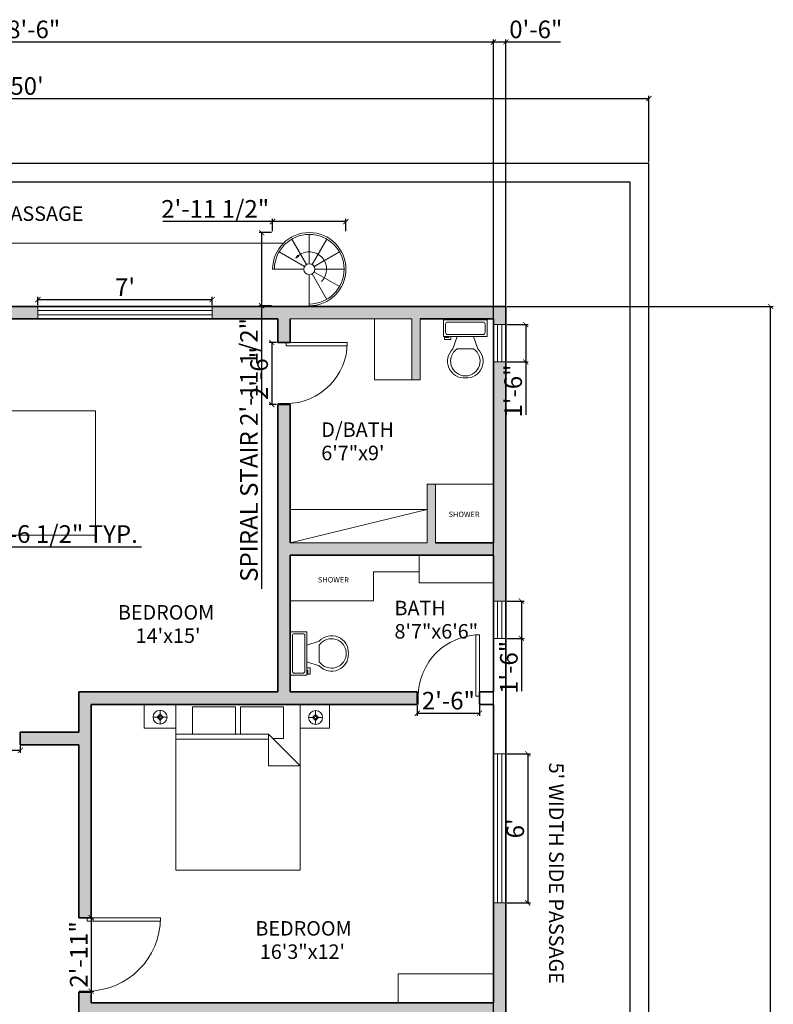
# Model space of a CAD drawing. Units: inches. Extents: x 3799 to 20199, y 1682 to 8087.
# Tile 13 of 30: x 11315 to 11679, y 2798 to 3273. Entities that reach past the tile are written whole.
import ezdxf

# ---------------------------------------------------------------- set-up
doc = ezdxf.new("R2010")
doc.units = ezdxf.units.IN
for name, color, linetype, lineweight in [('A-ANNO-DIMS', 2, 'Continuous', 18), ('A-ANNO-TEXT', 7, 'Continuous', 18), ('A-AREA-IDEN', 7, 'Continuous', 18), ('A-DOOR', 3, 'Continuous', 18), ('A-FLOR-CASE', 32, 'Continuous', 18), ('A-FLOR-FIXT', 9, 'Continuous', 18), ('A-FLOR-STRS', 41, 'Continuous', 18), ('A-FURN', 8, 'Continuous', 18), ('A-GLAZ', 152, 'Continuous', 18), ('A-WALL', 7, 'Continuous', 35), ('A-WALL-PATT', 252, 'Continuous', 13), ('C-PROP', 7, 'Continuous', 25)]:
    doc.layers.add(name, color=color, linetype=linetype, lineweight=lineweight)
doc.styles.get("Standard").update_dxf_attribs({"font": 'arial.ttf'})
doc.dimstyles.new('ISO-25', dxfattribs={"dimtxt": 8.5, "dimasz": 2.5, "dimexe": 1.25, "dimexo": 0.625, "dimtad": 1, "dimdec": 0, "dimlunit": 3, "dimtxsty": 'Standard', "dimblk": 'ARCHTICK', "dimcen": 2.5, "dimadec": 0, "dimazin": 0, "dimtfac": 1, "dimtdec": 0, "dimtmove": 0, "dimatfit": 3, "dimfxl": 1, "dimarcsym": 0})

# ---------------------------------------------------------------- blocks, each defined once
blk = doc.blocks.new('Bed - Queen')
for p, q in [((0, -80.00003), (0, 0)), ((0, 0), (59.99999, 0)), ((59.99999, 0), (59.99999, -80.00003)), ((7.99999, -1.2), (28.79998, -1.2)), ((7.99999, -14.4), (7.99999, -1.2)), ((28.79998, -1.2), (28.79998, -14.4)), ((31.19999, -1.2), (51.99999, -1.2)), ((31.19999, -14.4), (31.19999, -1.2)), ((51.99999, -1.2), (51.99999, -16.4)), ((0, -14.4), (44.8, -14.4)), ((44.8, -16.8), (0, -16.8)), ((59.99999, -29.6), (44.8, -14.4)), ((44.8, -14.4), (44.8, -29.6)), ((51.99999, -16.4), (46.79936, -16.4)), ((44.8, -29.6), (59.99999, -29.6)), ((59.99999, -80.00003), (0, -80.00003))]:
    blk.add_line(p, q)
blk = doc.blocks.new('*U59')
for p, q in [((9.5, -6), (9.5, -2)), ((-10, -8.5), (-8, -8.5)), ((-10, -9.5), (-10, -8.5)), ((-7, -9.5), (-10, -9.5)), ((-8, -8.5), (-8, -8)), ((-7, -8), (-7, -9.5)), ((-4, -8), (-6, -14)), ((4, -8), (6, -14)), ((4, -14), (-4, -14))]:
    blk.add_line(p, q)
blk.add_lwpolyline([(10.5, -8), (10.5, 0), (-10.5, 0), (-10.5, -8)], close=True)
for points in [[(-9.5, -2), (-9.5, -6)], [(8.5, -1), (-8.5, -1)], [(-8.5, -7), (8.5, -7)]]:
    blk.add_lwpolyline(points)
for centre, radius, start, end in [((-8.625, -1.875), 0.8839, 81.8699, 188.1301), ((8.625, -1.875), 0.8839, 351.8699, 98.1301), ((-8.625, -6.125), 0.8839, 171.869898, 278.1301), ((8.625, -6.125), 0.8839, 261.8699, 8.1301), ((-0.4772, -19.9188), 8.0953, 133.01722, 273.38), ((0.0374, -19.8731), 7.127, 124.50543, 269.7), ((-0.0373, -19.8731), 7.127, 270.3, 55.4946), ((0.4773, -19.9188), 8.0953, 266.62, 46.9828)]:
    blk.add_arc(centre, radius, start, end)
blk = doc.blocks.new('*U47')
for p, q in [((0, 0), (0, -100)), ((750, 0), (750, -100))]:
    blk.add_line(p, q)
blk.add_lwpolyline([(0, 0), (0, 750), (43.75, 750), (43.75, 0)], close=True)
blk.add_arc((0, 0), 750, 0, 90)
blk = doc.blocks.new('*U48')
for p, q in [((-750, 0), (-750, -100)), ((0, 0), (0, -100))]:
    blk.add_line(p, q)
blk.add_lwpolyline([(0, 0), (0, 750), (-43.75, 750), (-43.75, 0)], close=True)
blk.add_arc((0, 0), 750, 90, 180)
blk = doc.blocks.new('*U51')
for p, q in [((0, 0), (0, -100)), ((900, 0), (900, -100))]:
    blk.add_line(p, q)
blk.add_lwpolyline([(0, 0), (0, 900), (43.75, 900), (43.75, 0)], close=True)
blk.add_arc((0, 0), 900, 0, 90)
blk = doc.blocks.new('_ArchTick')
at = {"color": 0, "linetype": 'ByBlock', "const_width": 0.15}
blk.add_lwpolyline([(-0.5, -0.5), (0.5, 0.5)], dxfattribs=at)
blk = doc.blocks.new('*D65')
at = {"layer": 'A-ANNO-DIMS', "color": 0, "lineweight": -2, "transparency": 16777216}
for p, q in [((11324.12, 3135.7), (11324.12, 3139.65)), ((11324.12, 3138.4), (11408.12, 3138.4)), ((11408.12, 3135.7), (11408.12, 3139.65))]:
    blk.add_line(p, q, dxfattribs=at)
at = {"layer": 'Defpoints', "color": 0, "transparency": 16777216}
for p in [(11408.12, 3138.4), (11324.12, 3135.07), (11408.12, 3135.07)]:
    blk.add_point(p, dxfattribs=at)
at = {"layer": 'A-ANNO-DIMS', "color": 0, "lineweight": -2, "transparency": 16777216, "xscale": 2.5, "yscale": 2.5, "zscale": 2.5, "rotation": 180}
blk.add_blockref('_ArchTick', (11324.12, 3138.4), dxfattribs=at)
at = {"layer": 'A-ANNO-DIMS', "color": 0, "lineweight": -2, "transparency": 16777216, "xscale": 2.5, "yscale": 2.5, "zscale": 2.5}
blk.add_blockref('_ArchTick', (11408.12, 3138.4), dxfattribs=at)
at = {"layer": 'A-ANNO-DIMS', "color": 0, "transparency": 16777216, "insert": (11366.12, 3143.28), "char_height": 8.5, "attachment_point": 5}
blk.add_mtext("7'", dxfattribs=at)
blk = doc.blocks.new('*D66')
at = {"layer": 'A-ANNO-DIMS', "color": 0, "lineweight": -2, "transparency": 16777216}
for p, q in [((11550.48, 3126.28), (11560.66, 3126.28)), ((11559.41, 3126.28), (11559.41, 3108.28)), ((11550.48, 3108.28), (11560.66, 3108.28)), ((11559.41, 3108.28), (11559.41, 3082.73))]:
    blk.add_line(p, q, dxfattribs=at)
at = {"layer": 'Defpoints', "color": 0, "transparency": 16777216}
for p in [(11549.85, 3126.28), (11549.85, 3108.28), (11559.41, 3108.28)]:
    blk.add_point(p, dxfattribs=at)
at = {"layer": 'A-ANNO-DIMS', "color": 0, "lineweight": -2, "transparency": 16777216, "xscale": 2.5, "yscale": 2.5, "zscale": 2.5}
for p, rotation in [((11559.41, 3126.28), 90), ((11559.41, 3108.28), 270)]:
    blk.add_blockref('_ArchTick', p, dxfattribs=dict(at, rotation=rotation))
at = {"layer": 'A-ANNO-DIMS', "color": 0, "transparency": 16777216, "insert": (11554.45, 3094.25), "char_height": 8.5, "attachment_point": 5, "rotation": 90}
blk.add_mtext('1\'-6"', dxfattribs=at)
blk = doc.blocks.new('*D67')
at = {"layer": 'A-ANNO-DIMS', "color": 0, "lineweight": -2, "transparency": 16777216}
for p, q in [((11550.48, 2992.92), (11558.6, 2992.92)), ((11557.35, 2992.92), (11557.35, 2974.92)), ((11550.48, 2974.92), (11558.6, 2974.92)), ((11557.35, 2974.92), (11557.35, 2949.38))]:
    blk.add_line(p, q, dxfattribs=at)
at = {"layer": 'Defpoints', "color": 0, "transparency": 16777216}
for p in [(11549.85, 2992.92), (11549.85, 2974.92), (11557.35, 2974.92)]:
    blk.add_point(p, dxfattribs=at)
at = {"layer": 'A-ANNO-DIMS', "color": 0, "lineweight": -2, "transparency": 16777216, "xscale": 2.5, "yscale": 2.5, "zscale": 2.5}
for p, rotation in [((11557.35, 2992.92), 90), ((11557.35, 2974.92), 270)]:
    blk.add_blockref('_ArchTick', p, dxfattribs=dict(at, rotation=rotation))
at = {"layer": 'A-ANNO-DIMS', "color": 0, "transparency": 16777216, "insert": (11552.38, 2960.9), "char_height": 8.5, "attachment_point": 5, "rotation": 90}
blk.add_mtext('1\'-6"', dxfattribs=at)
blk = doc.blocks.new('*D68')
at = {"layer": 'A-ANNO-DIMS', "color": 0, "lineweight": -2, "transparency": 16777216}
for p, q in [((11550.48, 2919.23), (11561.66, 2919.23)), ((11560.41, 2919.23), (11560.41, 2847.23)), ((11550.48, 2847.23), (11561.66, 2847.23))]:
    blk.add_line(p, q, dxfattribs=at)
at = {"layer": 'Defpoints', "color": 0, "transparency": 16777216}
for p in [(11549.85, 2919.23), (11549.85, 2847.23), (11560.41, 2847.23)]:
    blk.add_point(p, dxfattribs=at)
at = {"layer": 'A-ANNO-DIMS', "color": 0, "lineweight": -2, "transparency": 16777216, "xscale": 2.5, "yscale": 2.5, "zscale": 2.5}
for p, rotation in [((11560.41, 2919.23), 90), ((11560.41, 2847.23), 270)]:
    blk.add_blockref('_ArchTick', p, dxfattribs=dict(at, rotation=rotation))
at = {"layer": 'A-ANNO-DIMS', "color": 0, "transparency": 16777216, "insert": (11555.45, 2883.23), "char_height": 8.5, "attachment_point": 5, "rotation": 90}
blk.add_mtext("6'", dxfattribs=at)
blk = doc.blocks.new('*D78')
at = {"layer": 'A-ANNO-DIMS', "color": 0, "lineweight": -2, "transparency": 16777216}
for p, q in [((11018.85, 3204.7), (11018.85, 3236.64)), ((11618.85, 3204.7), (11618.85, 3236.64)), ((11018.85, 3235.39), (11618.85, 3235.39))]:
    blk.add_line(p, q, dxfattribs=at)
at = {"layer": 'Defpoints', "color": 0, "transparency": 16777216}
for p in [(11618.85, 3235.39), (11018.85, 3204.07), (11618.85, 3204.07)]:
    blk.add_point(p, dxfattribs=at)
at = {"layer": 'A-ANNO-DIMS', "color": 0, "lineweight": -2, "transparency": 16777216, "xscale": 2.5, "yscale": 2.5, "zscale": 2.5, "rotation": 180}
blk.add_blockref('_ArchTick', (11018.85, 3235.39), dxfattribs=at)
at = {"layer": 'A-ANNO-DIMS', "color": 0, "lineweight": -2, "transparency": 16777216, "xscale": 2.5, "yscale": 2.5, "zscale": 2.5}
blk.add_blockref('_ArchTick', (11618.85, 3235.39), dxfattribs=at)
at = {"layer": 'A-ANNO-DIMS', "color": 0, "transparency": 16777216, "insert": (11318.85, 3240.35), "char_height": 8.5, "attachment_point": 5}
blk.add_mtext("50'", dxfattribs=at)
blk = doc.blocks.new('*D84')
at = {"layer": 'A-ANNO-DIMS', "color": 0, "lineweight": -2, "transparency": 16777216}
for p, q in [((11344.48, 2840.12), (11351.04, 2840.12)), ((11349.79, 2840.12), (11349.79, 2804.68)), ((11344.48, 2804.68), (11351.04, 2804.68))]:
    blk.add_line(p, q, dxfattribs=at)
at = {"layer": 'Defpoints', "color": 0, "transparency": 16777216}
for p in [(11343.85, 2840.12), (11343.85, 2804.68), (11349.79, 2804.68)]:
    blk.add_point(p, dxfattribs=at)
at = {"layer": 'A-ANNO-DIMS', "color": 0, "lineweight": -2, "transparency": 16777216, "xscale": 2.5, "yscale": 2.5, "zscale": 2.5}
for p, rotation in [((11349.79, 2840.12), 90), ((11349.79, 2804.68), 270)]:
    blk.add_blockref('_ArchTick', p, dxfattribs=dict(at, rotation=rotation))
at = {"layer": 'A-ANNO-DIMS', "color": 0, "transparency": 16777216, "insert": (11344.9, 2822.4), "char_height": 8.5, "attachment_point": 5, "rotation": 90}
blk.add_mtext('2\'-11"', dxfattribs=at)
blk = doc.blocks.new('*D86')
at = {"layer": 'A-ANNO-DIMS', "color": 0, "lineweight": -2, "transparency": 16777216}
for p, q in [((11279.6, 2922.98), (11279.6, 2919.65)), ((11315.6, 2922.98), (11315.6, 2919.65)), ((11279.6, 2920.9), (11315.6, 2920.9))]:
    blk.add_line(p, q, dxfattribs=at)
at = {"layer": 'Defpoints', "color": 0, "transparency": 16777216}
for p in [(11279.6, 2923.61), (11315.6, 2923.61), (11315.6, 2920.9)]:
    blk.add_point(p, dxfattribs=at)
at = {"layer": 'A-ANNO-DIMS', "color": 0, "lineweight": -2, "transparency": 16777216, "xscale": 2.5, "yscale": 2.5, "zscale": 2.5, "rotation": 180}
blk.add_blockref('_ArchTick', (11279.6, 2920.9), dxfattribs=at)
at = {"layer": 'A-ANNO-DIMS', "color": 0, "lineweight": -2, "transparency": 16777216, "xscale": 2.5, "yscale": 2.5, "zscale": 2.5}
blk.add_blockref('_ArchTick', (11315.6, 2920.9), dxfattribs=at)
at = {"layer": 'A-ANNO-DIMS', "color": 0, "transparency": 16777216, "insert": (11297.6, 2925.87), "char_height": 8.5, "attachment_point": 5}
blk.add_mtext("3'", dxfattribs=at)
blk = doc.blocks.new('*D88')
at = {"layer": 'A-ANNO-DIMS', "color": 0, "lineweight": -2, "transparency": 16777216}
for p, q in [((11507.11, 2942.45), (11507.11, 2937.53)), ((11537.11, 2942.45), (11537.11, 2937.53)), ((11507.11, 2938.78), (11537.11, 2938.78))]:
    blk.add_line(p, q, dxfattribs=at)
at = {"layer": 'Defpoints', "color": 0, "transparency": 16777216}
for p in [(11507.11, 2943.07), (11537.11, 2943.07), (11537.11, 2938.78)]:
    blk.add_point(p, dxfattribs=at)
at = {"layer": 'A-ANNO-DIMS', "color": 0, "lineweight": -2, "transparency": 16777216, "xscale": 2.5, "yscale": 2.5, "zscale": 2.5, "rotation": 180}
blk.add_blockref('_ArchTick', (11507.11, 2938.78), dxfattribs=at)
at = {"layer": 'A-ANNO-DIMS', "color": 0, "lineweight": -2, "transparency": 16777216, "xscale": 2.5, "yscale": 2.5, "zscale": 2.5}
blk.add_blockref('_ArchTick', (11537.11, 2938.78), dxfattribs=at)
at = {"layer": 'A-ANNO-DIMS', "color": 0, "transparency": 16777216, "insert": (11522.11, 2943.74), "char_height": 8.5, "attachment_point": 5}
blk.add_mtext('2\'-6"', dxfattribs=at)
blk = doc.blocks.new('*D89')
at = {"layer": 'A-ANNO-DIMS', "color": 0, "lineweight": -2, "transparency": 16777216}
for p, q in [((11439.23, 3117.71), (11435.63, 3117.71)), ((11436.88, 3117.71), (11436.88, 3087.71)), ((11439.23, 3087.71), (11435.63, 3087.71))]:
    blk.add_line(p, q, dxfattribs=at)
at = {"layer": 'Defpoints', "color": 0, "transparency": 16777216}
for p in [(11439.85, 3117.71), (11436.88, 3087.71), (11439.85, 3087.71)]:
    blk.add_point(p, dxfattribs=at)
at = {"layer": 'A-ANNO-DIMS', "color": 0, "lineweight": -2, "transparency": 16777216, "xscale": 2.5, "yscale": 2.5, "zscale": 2.5}
for p, rotation in [((11436.88, 3117.71), 90), ((11436.88, 3087.71), 270)]:
    blk.add_blockref('_ArchTick', p, dxfattribs=dict(at, rotation=rotation))
at = {"layer": 'A-ANNO-DIMS', "color": 0, "transparency": 16777216, "insert": (11431.91, 3102.71), "char_height": 8.5, "attachment_point": 5, "rotation": 90}
blk.add_mtext('2\'-6"', dxfattribs=at)
blk = doc.blocks.new('Lamp - Table')
for p, q in [((-1, 0), (-7, 0)), ((0, 3), (-3, 0)), ((-3, 0), (0, -3)), ((0, 7), (0, 1)), ((3, 0), (0, 3)), ((0, -3), (3, 0)), ((1, 0), (7, 0)), ((0, -1), (0, -7))]:
    blk.add_line(p, q)
for radius in [7, 1]:
    blk.add_circle((0, 0), radius)
blk = doc.blocks.new('Staircase - Spiral')
for p, q in [((-2.2579, 3.91), (-14.25, 24.681)), ((0, 4.5), (0, 30)), ((-3.8566, 2.226), (-24.6818, 14.25)), ((-4.5, 0), (-28.5, 0)), ((4.5, 0), (30, 0)), ((-3.8954, -2.2492), (-24.6818, -14.2502)), ((-2.2755, -3.9415), (-14.25, -24.6819)), ((0, -4.5002), (0, -28.5002)), ((2.2614, -3.9171), (14.25, -24.6819)), ((3.8999, -2.2518), (24.6817, -14.2502)), ((8.5, -10.5002), (11, -9.0002)), ((9, -11.0002), (8.5, -10.5002)), ((9, -11.0002), (9.5, -11.5002)), ((11, -9.0002), (9.5, -11.5002))]:
    blk.add_line(p, q)
blk.add_circle((0, 0), 4.5)
for radius, start, end in [(30, 90, 0), (28.5, 90, 0), (14.2215, 135, 309.2894)]:
    blk.add_arc((0, 0), radius, start, end)
blk = doc.blocks.new('WIN-84IN-6IN-FRAME')
for p, q in [((0, 84), (6, 84)), ((2, 0), (2, 84)), ((4, 0), (4, 84)), ((0, 0), (6, 0))]:
    blk.add_line(p, q)
blk = doc.blocks.new('WIN-18IN-6IN-FRAME')
for p, q in [((0, 18), (6, 18)), ((2, 0), (2, 18)), ((4, 0), (4, 18)), ((0, 0), (6, 0))]:
    blk.add_line(p, q)
blk = doc.blocks.new('*D246')
at = {"layer": 'A-ANNO-DIMS', "color": 0, "lineweight": -2, "transparency": 16777216}
for p, q in [((11256.67, 3019.5), (11256.67, 3017.87)), ((11256.67, 3019.12), (11263.41, 3019.12)), ((11263.41, 3019.5), (11263.41, 3017.87)), ((11263.41, 3019.12), (11374.03, 3019.12))]:
    blk.add_line(p, q, dxfattribs=at)
at = {"layer": 'Defpoints', "color": 0, "transparency": 16777216}
for p in [(11256.67, 3020.13), (11263.41, 3020.13), (11263.41, 3019.12)]:
    blk.add_point(p, dxfattribs=at)
at = {"layer": 'A-ANNO-DIMS', "color": 0, "lineweight": -2, "transparency": 16777216, "xscale": 2.5, "yscale": 2.5, "zscale": 2.5, "rotation": 180}
blk.add_blockref('_ArchTick', (11256.67, 3019.12), dxfattribs=at)
at = {"layer": 'A-ANNO-DIMS', "color": 0, "lineweight": -2, "transparency": 16777216, "xscale": 2.5, "yscale": 2.5, "zscale": 2.5}
blk.add_blockref('_ArchTick', (11263.41, 3019.12), dxfattribs=at)
at = {"layer": 'A-ANNO-DIMS', "color": 0, "transparency": 16777216, "insert": (11319.97, 3024.14), "char_height": 8.5, "attachment_point": 5}
blk.add_mtext('LAMP 0\'-6 1/2" TYP.', dxfattribs=at)
blk = doc.blocks.new('*D350')
at = {"layer": 'A-ANNO-DIMS', "color": 0, "lineweight": -2, "transparency": 16777216}
for p, q in [((11436.7, 3170.72), (11430.77, 3170.72)), ((11432.02, 3170.72), (11432.02, 3135.36)), ((11436.7, 3135.36), (11430.77, 3135.36)), ((11432.02, 3135.36), (11432.02, 2998.84))]:
    blk.add_line(p, q, dxfattribs=at)
at = {"layer": 'Defpoints', "color": 0, "transparency": 16777216}
for p in [(11437.32, 3170.72), (11432.02, 3135.36), (11437.32, 3135.36)]:
    blk.add_point(p, dxfattribs=at)
at = {"layer": 'A-ANNO-DIMS', "color": 0, "lineweight": -2, "transparency": 16777216, "xscale": 2.5, "yscale": 2.5, "zscale": 2.5}
for p, rotation in [((11432.02, 3170.72), 90), ((11432.02, 3135.36), 270)]:
    blk.add_blockref('_ArchTick', p, dxfattribs=dict(at, rotation=rotation))
at = {"layer": 'A-ANNO-DIMS', "color": 0, "transparency": 16777216, "insert": (11427, 3065.85), "char_height": 8.5, "attachment_point": 5, "rotation": 90}
blk.add_mtext('SPIRAL STAIR 2\'-11 1/2"', dxfattribs=at)
blk = doc.blocks.new('*D351')
at = {"layer": 'A-ANNO-DIMS', "color": 0, "lineweight": -2, "transparency": 16777216}
for p, q in [((11437.32, 3176.02), (11384.42, 3176.02)), ((11437.32, 3171.34), (11437.32, 3177.27)), ((11472.68, 3176.02), (11437.32, 3176.02)), ((11472.68, 3171.34), (11472.68, 3177.27))]:
    blk.add_line(p, q, dxfattribs=at)
at = {"layer": 'Defpoints', "color": 0, "transparency": 16777216}
for p in [(11437.32, 3176.02), (11437.32, 3170.72), (11472.68, 3170.72)]:
    blk.add_point(p, dxfattribs=at)
at = {"layer": 'A-ANNO-DIMS', "color": 0, "lineweight": -2, "transparency": 16777216, "xscale": 2.5, "yscale": 2.5, "zscale": 2.5, "rotation": 180}
blk.add_blockref('_ArchTick', (11437.32, 3176.02), dxfattribs=at)
at = {"layer": 'A-ANNO-DIMS', "color": 0, "lineweight": -2, "transparency": 16777216, "xscale": 2.5, "yscale": 2.5, "zscale": 2.5}
blk.add_blockref('_ArchTick', (11472.68, 3176.02), dxfattribs=at)
at = {"layer": 'A-ANNO-DIMS', "color": 0, "transparency": 16777216, "insert": (11409.62, 3181.04), "char_height": 8.5, "attachment_point": 5}
blk.add_mtext('2\'-11 1/2"', dxfattribs=at)
blk = doc.blocks.new('*D371')
at = {"layer": 'A-ANNO-DIMS', "color": 0, "lineweight": -2, "transparency": 16777216}
for p, q in [((11543.85, 3126.9), (11543.85, 3263.92)), ((11549.85, 3126.9), (11549.85, 3263.92)), ((11543.85, 3262.67), (11549.85, 3262.67)), ((11549.85, 3262.67), (11576.2, 3262.67))]:
    blk.add_line(p, q, dxfattribs=at)
at = {"layer": 'Defpoints', "color": 0, "transparency": 16777216}
for p in [(11549.85, 3262.67), (11543.85, 3126.28), (11549.85, 3126.28)]:
    blk.add_point(p, dxfattribs=at)
at = {"layer": 'A-ANNO-DIMS', "color": 0, "lineweight": -2, "transparency": 16777216, "xscale": 2.5, "yscale": 2.5, "zscale": 2.5, "rotation": 180}
blk.add_blockref('_ArchTick', (11543.85, 3262.67), dxfattribs=at)
at = {"layer": 'A-ANNO-DIMS', "color": 0, "lineweight": -2, "transparency": 16777216, "xscale": 2.5, "yscale": 2.5, "zscale": 2.5}
blk.add_blockref('_ArchTick', (11549.85, 3262.67), dxfattribs=at)
at = {"layer": 'A-ANNO-DIMS', "color": 0, "transparency": 16777216, "insert": (11564.28, 3267.64), "char_height": 8.5, "attachment_point": 5}
blk.add_mtext('0\'-6"', dxfattribs=at)
blk = doc.blocks.new('*D372')
at = {"layer": 'A-ANNO-DIMS', "color": 0, "lineweight": -2, "transparency": 16777216}
for p, q in [((11543.85, 2537.7), (11543.85, 3263.92)), ((11549.85, 2537.7), (11549.85, 3263.92)), ((11543.85, 3262.67), (11549.85, 3262.67)), ((11549.85, 3262.67), (11576.2, 3262.67))]:
    blk.add_line(p, q, dxfattribs=at)
at = {"layer": 'Defpoints', "color": 0, "transparency": 16777216}
for p in [(11549.85, 3262.67), (11543.85, 2537.07), (11549.85, 2537.07)]:
    blk.add_point(p, dxfattribs=at)
at = {"layer": 'A-ANNO-DIMS', "color": 0, "lineweight": -2, "transparency": 16777216, "xscale": 2.5, "yscale": 2.5, "zscale": 2.5, "rotation": 180}
blk.add_blockref('_ArchTick', (11543.85, 3262.67), dxfattribs=at)
at = {"layer": 'A-ANNO-DIMS', "color": 0, "lineweight": -2, "transparency": 16777216, "xscale": 2.5, "yscale": 2.5, "zscale": 2.5}
blk.add_blockref('_ArchTick', (11549.85, 3262.67), dxfattribs=at)
at = {"layer": 'A-ANNO-DIMS', "color": 0, "transparency": 16777216, "insert": (11564.28, 3267.64), "char_height": 8.5, "attachment_point": 5}
blk.add_mtext('0\'-6"', dxfattribs=at)
blk = doc.blocks.new('*D373')
at = {"layer": 'A-ANNO-DIMS', "color": 0, "lineweight": -2, "transparency": 16777216}
for p, q in [((11087.85, 3135.7), (11087.85, 3263.92)), ((11549.85, 3135.7), (11549.85, 3263.92)), ((11087.85, 3262.67), (11549.85, 3262.67))]:
    blk.add_line(p, q, dxfattribs=at)
at = {"layer": 'Defpoints', "color": 0, "transparency": 16777216}
for p in [(11549.85, 3262.67), (11087.85, 3135.07), (11549.85, 3135.07)]:
    blk.add_point(p, dxfattribs=at)
at = {"layer": 'A-ANNO-DIMS', "color": 0, "lineweight": -2, "transparency": 16777216, "xscale": 2.5, "yscale": 2.5, "zscale": 2.5, "rotation": 180}
blk.add_blockref('_ArchTick', (11087.85, 3262.67), dxfattribs=at)
at = {"layer": 'A-ANNO-DIMS', "color": 0, "lineweight": -2, "transparency": 16777216, "xscale": 2.5, "yscale": 2.5, "zscale": 2.5}
blk.add_blockref('_ArchTick', (11549.85, 3262.67), dxfattribs=at)
at = {"layer": 'A-ANNO-DIMS', "color": 0, "transparency": 16777216, "insert": (11318.85, 3267.64), "char_height": 8.5, "attachment_point": 5}
blk.add_mtext('38\'-6"', dxfattribs=at)
blk = doc.blocks.new('*D374')
at = {"layer": 'A-ANNO-DIMS', "color": 0, "lineweight": -2, "transparency": 16777216}
for p, q in [((11550.48, 3135.07), (11678.7, 3135.07)), ((11677.45, 2325.07), (11677.45, 3135.07)), ((11550.48, 2325.07), (11678.7, 2325.07))]:
    blk.add_line(p, q, dxfattribs=at)
at = {"layer": 'Defpoints', "color": 0, "transparency": 16777216}
for p in [(11549.85, 3135.07), (11677.45, 3135.07), (11549.85, 2325.07)]:
    blk.add_point(p, dxfattribs=at)
at = {"layer": 'A-ANNO-DIMS', "color": 0, "lineweight": -2, "transparency": 16777216, "xscale": 2.5, "yscale": 2.5, "zscale": 2.5}
for p, rotation in [((11677.45, 3135.07), 90), ((11677.45, 2325.07), 270)]:
    blk.add_blockref('_ArchTick', p, dxfattribs=dict(at, rotation=rotation))
at = {"layer": 'A-ANNO-DIMS', "color": 0, "transparency": 16777216, "insert": (11672.49, 2730.07), "char_height": 8.5, "attachment_point": 5, "rotation": 90}
blk.add_mtext('67\'-6"', dxfattribs=at)

msp = doc.modelspace()

# ---------------------------------------------------------------- hatches: boundary and pattern name
at = {"layer": 'A-WALL-PATT'}
h = msp.add_hatch(color=256, dxfattribs=at)
h.dxf.hatch_style = 1
h.paths.add_polyline_path([(11549.85, 2537.07), (11543.85, 2537.07), (11543.85, 2493.07), (11500.92, 2493.07), (11500.92, 2487.07), (11543.85, 2487.07), (11543.85, 2331.07), (11512.59, 2331.07), (11512.59, 2325.07), (11549.85, 2325.07)])
h.paths.add_polyline_path([(11404.92, 2493.07), (11369.85, 2493.07), (11369.85, 2535.29), (11363.85, 2535.29), (11363.85, 2493.07), (11359.67, 2493.07), (11359.67, 2487.07), (11404.92, 2487.07)])
h.paths.add_polyline_path([(11347.67, 2493.07), (11315.85, 2493.07), (11315.85, 2481.32), (11321.85, 2481.32), (11321.85, 2487.07), (11347.67, 2487.07)])
h.paths.add_polyline_path([(11246.96, 2394.07), (11231.85, 2394.07), (11231.85, 2493.07), (11126.81, 2493.07), (11126.81, 2487.07), (11225.85, 2487.07), (11225.85, 2325.07), (11315.85, 2325.07), (11315.85, 2331.07), (11231.85, 2331.07), (11231.85, 2388.07), (11246.96, 2388.07)])
h.paths.add_polyline_path([(11368.59, 2331.07), (11321.85, 2331.07), (11321.85, 2421.32), (11319.79, 2421.32), (11315.85, 2421.32), (11315.85, 2394.07), (11306.96, 2394.07), (11306.96, 2392.01), (11306.96, 2388.07), (11315.85, 2388.07), (11315.85, 2325.07), (11368.59, 2325.07)])
h.paths.add_polyline_path([(11211.5, 2599.62), (11175.25, 2599.62), (11175.25, 2594.62), (11206.5, 2594.62), (11206.5, 2541.62), (11137.5, 2541.62), (11137.5, 2594.62), (11145.25, 2594.62), (11145.25, 2599.62), (11132.5, 2599.62), (11132.5, 2536.62), (11211.5, 2536.62)], flags=17)
h.paths.add_polyline_path([(11278.96, 2650.07), (11117.85, 2650.07), (11117.85, 2668.07), (11111.85, 2668.07), (11111.85, 2650.07), (11087.85, 2650.07), (11087.85, 2526.57), (11093.85, 2526.57), (11093.85, 2644.07), (11278.96, 2644.07)])
h.paths.add_polyline_path([(11096.81, 2491.01), (11096.81, 2493.07), (11093.85, 2493.07), (11093.85, 2496.57), (11087.85, 2496.57), (11087.85, 2487.07), (11096.81, 2487.07)])
h.paths.add_polyline_path([(11445.85, 3087.71), (11439.85, 3087.71), (11439.85, 2949.07), (11343.85, 2949.07), (11343.85, 2929.61), (11315.6, 2929.61), (11315.6, 2923.61), (11343.85, 2923.61), (11343.85, 2840.12), (11349.85, 2840.12), (11349.85, 2943.07), (11507.11, 2943.07), (11507.11, 2949.07), (11445.85, 2949.07), (11445.85, 3015.07), (11543.85, 3015.07), (11543.85, 2992.92), (11549.85, 2992.92), (11549.85, 3108.28), (11543.85, 3108.28), (11543.85, 3021.07), (11515.89, 3021.07), (11515.89, 3049.36), (11511.89, 3049.36), (11511.89, 3021.07), (11445.85, 3021.07)])
h.paths.add_polyline_path([(11549.85, 3135.07), (11408.12, 3135.07), (11408.12, 3129.07), (11439.85, 3129.07), (11439.85, 3117.71), (11443.79, 3117.71), (11445.85, 3117.71), (11445.85, 3129.07), (11504.47, 3129.07), (11504.47, 3099.65), (11508.47, 3099.65), (11508.47, 3129.07), (11543.85, 3129.07), (11543.85, 3126.28), (11549.85, 3126.28)])
h.paths.add_polyline_path([(11324.12, 3135.07), (11087.85, 3135.07), (11087.85, 3083.46), (11093.85, 3083.46), (11093.85, 3129.07), (11265.85, 3129.07), (11265.85, 3050.07), (11240.75, 3050.07), (11240.75, 3044.07), (11265.85, 3044.07), (11265.85, 2895.64), (11271.85, 2895.64), (11271.85, 2923.61), (11279.6, 2923.61), (11279.6, 2929.61), (11271.85, 2929.61), (11271.85, 3129.07), (11324.12, 3129.07)])
h.paths.add_polyline_path([(11210.75, 3050.07), (11133.85, 3050.07), (11133.85, 3088.63), (11129.85, 3088.54), (11129.85, 3050.07), (11093.85, 3050.07), (11093.85, 3059.46), (11087.85, 3059.46), (11087.85, 3030.25), (11093.85, 3030.25), (11093.85, 3044.07), (11210.75, 3044.07)], flags=17)
h.paths.add_polyline_path([(11093.85, 2982.25), (11087.85, 2982.25), (11087.85, 2913.95), (11093.85, 2913.95)], flags=17)
h.paths.add_polyline_path([(11271.85, 2859.64), (11265.85, 2859.64), (11265.85, 2854.07), (11093.85, 2854.07), (11093.85, 2865.95), (11087.85, 2865.95), (11087.85, 2848.07), (11111.85, 2848.07), (11111.85, 2812.07), (11117.85, 2812.07), (11117.85, 2848.07), (11271.85, 2848.07)])
h.paths.add_polyline_path([(11549.85, 2847.23), (11543.85, 2847.23), (11543.85, 2799.07), (11349.85, 2799.07), (11349.85, 2804.12), (11343.85, 2804.12), (11343.85, 2753.07), (11349.85, 2753.07), (11349.85, 2793.07), (11543.85, 2793.07), (11543.85, 2752.31), (11549.85, 2752.31)])
h.paths.add_polyline_path([(11549.85, 2692.31), (11543.85, 2692.31), (11543.85, 2650.07), (11343.85, 2650.07), (11338.96, 2650.07), (11338.96, 2644.07), (11349.85, 2644.07), (11363.85, 2644.07), (11363.85, 2608.29), (11369.85, 2608.29), (11369.85, 2644.07), (11543.85, 2644.07), (11543.85, 2621.07), (11549.85, 2621.07)])

# ---------------------------------------------------------------- linework, layer by layer
at = {"layer": 'A-FLOR-CASE'}
for p, q in [((11543.85, 2812.98), (11497.92, 2812.98)), ((11497.92, 2812.98), (11497.92, 2799.07))]:
    msp.add_line(p, q, dxfattribs=at)
at = {"layer": 'A-FLOR-FIXT'}
for p, q in [((11504.47, 3129.07), (11445.85, 3129.07)), ((11486.47, 3129.07), (11486.47, 3099.65)), ((11504.47, 3129.07), (11504.47, 3099.65)), ((11508.47, 3129.07), (11508.47, 3099.65)), ((11486.47, 3099.65), (11504.47, 3099.65)), ((11508.47, 3099.65), (11504.47, 3099.65)), ((11511.89, 3021.07), (11511.89, 3049.36)), ((11511.89, 3049.36), (11543.85, 3049.36)), ((11515.89, 3021.07), (11515.89, 3049.36)), ((11511.89, 3037.17), (11445.85, 3037.17)), ((11445.85, 3021.07), (11511.89, 3037.17)), ((11511.89, 3021.07), (11445.85, 3021.07)), ((11508.04, 3001.74), (11508.04, 3015.07)), ((11508.04, 3007.02), (11486.04, 3007.02)), ((11486.04, 3007.02), (11486.04, 2993.01)), ((11543.85, 3001.74), (11508.04, 3001.74)), ((11486.04, 2993.01), (11445.85, 2993.01))]:
    msp.add_line(p, q, dxfattribs=at)
at = {"layer": 'A-FLOR-STRS'}
msp.add_line((11087.85, 3165.66), (11442.62, 3165.66), dxfattribs=at)
at = {"layer": 'A-FURN'}
for points in [[(11390.6, 2943.07), (11375.38, 2943.07), (11375.38, 2931.5), (11390.6, 2931.5)], [(11450.6, 2943.07), (11464.72, 2943.07), (11464.72, 2931.5), (11450.6, 2931.5)]]:
    msp.add_lwpolyline(points, close=True, dxfattribs=at)
at = {"layer": 'A-GLAZ'}
for p, q in [((11543.85, 2919.23), (11549.85, 2919.23)), ((11545.85, 2847.23), (11545.85, 2919.23)), ((11547.85, 2847.23), (11547.85, 2919.23)), ((11543.85, 2847.23), (11549.85, 2847.23))]:
    msp.add_line(p, q, dxfattribs=at)
at = {"layer": 'A-WALL'}
for p, q in [((11549.85, 3135.07), (11087.85, 3135.07)), ((11549.85, 2325.07), (11549.85, 3135.07)), ((11439.85, 3129.07), (11271.85, 3129.07)), ((11439.85, 3129.07), (11439.85, 3117.71)), ((11445.85, 3129.07), (11445.85, 3117.71)), ((11543.85, 3129.07), (11508.47, 3129.07)), ((11543.85, 3021.07), (11543.85, 3129.07)), ((11439.85, 3117.71), (11445.85, 3117.71)), ((11439.85, 3087.71), (11445.85, 3087.71)), ((11439.85, 3087.71), (11439.85, 2949.07)), ((11445.85, 3087.71), (11445.85, 3021.07)), ((11543.85, 3021.07), (11515.89, 3021.07)), ((11543.85, 3015.07), (11445.85, 3015.07)), ((11445.85, 3015.07), (11445.85, 2949.07)), ((11543.85, 2949.07), (11543.85, 3015.07)), ((11439.85, 2949.07), (11343.85, 2949.07)), ((11343.85, 2929.61), (11343.85, 2949.07)), ((11445.85, 2949.07), (11507.11, 2949.07)), ((11507.11, 2943.07), (11507.11, 2949.07)), ((11537.11, 2943.07), (11537.11, 2949.07)), ((11537.11, 2949.07), (11543.85, 2949.07)), ((11349.85, 2840.12), (11349.85, 2943.07)), ((11507.11, 2943.07), (11349.85, 2943.07)), ((11543.85, 2943.07), (11537.11, 2943.07)), ((11543.85, 2799.07), (11543.85, 2943.07)), ((11343.85, 2929.61), (11315.6, 2929.61)), ((11315.6, 2929.61), (11315.6, 2923.61)), ((11343.85, 2923.61), (11315.6, 2923.61)), ((11343.85, 2840.12), (11343.85, 2923.61)), ((11349.85, 2840.12), (11343.85, 2840.12)), ((11349.85, 2804.12), (11343.85, 2804.12)), ((11343.85, 2753.07), (11343.85, 2804.12)), ((11349.85, 2799.07), (11349.85, 2804.12)), ((11543.85, 2799.07), (11349.85, 2799.07))]:
    msp.add_line(p, q, dxfattribs=at)
at = {"layer": 'C-PROP'}
for p, q in [((11618.85, 3204.07), (11018.85, 3204.07)), ((11618.85, 2124.07), (11618.85, 3204.07)), ((11609.85, 3195.07), (11027.85, 3195.07)), ((11609.85, 2133.07), (11609.85, 3195.07))]:
    msp.add_line(p, q, dxfattribs=at)

# ---------------------------------------------------------------- block references
at = {"layer": 'A-DOOR', "xscale": 0.0393700787401575, "yscale": 0.0393700787401575, "zscale": 0.0393700787401575, "rotation": 270}
for name, p in [('*U47', (11443.79, 3117.71)), ('*U51', (11347.79, 2840.12))]:
    msp.add_blockref(name, p, dxfattribs=at)
at = {"layer": 'A-DOOR', "xscale": 0.0393700787401575, "yscale": 0.0393700787401575, "zscale": 0.0393700787401575}
msp.add_blockref('*U48', (11537.11, 2947.01), dxfattribs=at)
at = {"layer": 'A-FLOR-FIXT'}
msp.add_blockref('*U59', (11530.29, 3128.55), dxfattribs=at)
at = {"layer": 'A-FLOR-FIXT', "rotation": 90}
msp.add_blockref('*U59', (11445.85, 2967.63), dxfattribs=at)
at = {"layer": 'A-FLOR-STRS', "xscale": 0.5892392521496895, "yscale": 0.5892392521496895, "zscale": 0.5892392521496895, "rotation": 180}
msp.add_blockref('Staircase - Spiral', (11455, 3153.04), dxfattribs=at)
at = {"layer": 'A-FURN', "rotation": 90}
msp.add_blockref('Bed - Queen', (11271.85, 3024.65), dxfattribs=at)
at = {"layer": 'A-FURN'}
msp.add_blockref('Bed - Queen', (11390.6, 2943.07), dxfattribs=at)
at = {"layer": 'A-FURN', "xscale": 0.4812244018485111, "yscale": 0.4812244018485111, "zscale": 0.4812244018485111}
for p in [(11383, 2936.86), (11458.07, 2936.74)]:
    msp.add_blockref('Lamp - Table', p, dxfattribs=at)
at = {"layer": 'A-GLAZ', "rotation": 90}
msp.add_blockref('WIN-84IN-6IN-FRAME', (11408.12, 3129.07), dxfattribs=at)
at = {"layer": 'A-GLAZ'}
for p in [(11543.85, 3108.28), (11543.85, 2974.92)]:
    msp.add_blockref('WIN-18IN-6IN-FRAME', p, dxfattribs=at)

# ---------------------------------------------------------------- texts
at = {"layer": 'A-ANNO-TEXT'}
for rotation, p in [(0.0019, (11239.28, 3176.34)), (270.0019, (11570.67, 2914.93))]:
    msp.add_text("5' WIDTH SIDE PASSAGE", height=7, rotation=rotation, dxfattribs=at).set_placement(p)
at = {"layer": 'A-AREA-IDEN'}
for s, height, p in [('D/BATH', 7, (11460.79, 3072.13)), ('6\'7"x9\'', 7, (11460.79, 3060.88)), ('SHOWER', 2.63, (11522.21, 3033.42)), ('SHOWER', 2.63, (11459.16, 3001.87)), ('BEDROOM', 7, (11362.69, 2983.96)), ('BATH', 7, (11496.1, 2986.05)), ("    14'x15'", 7, (11362.69, 2972.71)), ('8\'7"x6\'6"', 7, (11496.1, 2974.81)), ('BEDROOM', 7, (11429, 2831.48)), (' 16\'3"x12\'', 7, (11429, 2820.24))]:
    msp.add_text(s, height=height, rotation=0.0019, dxfattribs=at).set_placement(p)

# ---------------------------------------------------------------- dimensions: what is measured, and where the dimension line sits
at = {"layer": 'A-ANNO-DIMS'}
for base, p1, p2, override, picture, middle in [((11549.85, 3262.67), (11087.85, 3135.07), (11549.85, 3135.07), {"dimdec": 1, "dimlfac": 1, "dimrnd": 0, "dimzin": 1, "dimdsep": 46, "dimlunit": 4, "dimfrac": 2}, '*D373', (11318.85, 3267.64)), ((11549.85, 3262.67), (11543.85, 3126.28), (11549.85, 3126.28), {"dimdec": 1, "dimlfac": 1, "dimrnd": 0, "dimzin": 1, "dimdsep": 46, "dimlunit": 4, "dimfrac": 2}, '*D371', (11564.28, 3267.64)), ((11549.85, 3262.67), (11543.85, 2537.07), (11549.85, 2537.07), {"dimdec": 1, "dimlfac": 1, "dimrnd": 0, "dimzin": 1, "dimdsep": 46, "dimlunit": 4, "dimfrac": 2}, '*D372', (11564.28, 3267.64)), ((11618.85, 3235.39), (11018.85, 3204.07), (11618.85, 3204.07), {"dimclrd": 0, "dimclre": 0, "dimclrt": 0}, '*D78', (11318.85, 3240.35)), ((11408.12, 3138.4), (11324.12, 3135.07), (11408.12, 3135.07), {"dimclrd": 0, "dimclre": 0, "dimclrt": 0}, '*D65', (11366.12, 3143.28)), ((11537.11, 2938.78), (11507.11, 2943.07), (11537.11, 2943.07), {"dimclrd": 0, "dimclre": 0, "dimclrt": 0}, '*D88', (11522.11, 2943.74)), ((11315.6, 2920.9), (11279.6, 2923.61), (11315.6, 2923.61), {"dimclrd": 0, "dimclre": 0, "dimclrt": 0}, '*D86', (11297.6, 2925.87))]:
    dim = msp.add_linear_dim(base=base, p1=p1, p2=p2, dimstyle='ISO-25', override=override, dxfattribs=at)
    dim.commit()
    dim.dimension.update_dxf_attribs({"geometry": picture, "text_midpoint": middle})
for base, p1, p2, angle, override, picture, middle in [((11437.32, 3176.02), (11472.68, 3170.72), (11437.32, 3170.72), 180, {"dimdec": 1, "dimlfac": 1, "dimrnd": 0, "dimzin": 1, "dimdsep": 46, "dimlunit": 4, "dimfrac": 2}, '*D351', (11409.62, 3181.04)), ((11677.45, 3135.07), (11549.85, 2325.07), (11549.85, 3135.07), 90, {"dimdec": 1, "dimlfac": 1, "dimrnd": 0, "dimzin": 1, "dimdsep": 46, "dimlunit": 4, "dimfrac": 2}, '*D374', (11672.49, 2730.07)), ((11559.41, 3108.28), (11549.85, 3126.28), (11549.85, 3108.28), 90, {"dimclrd": 0, "dimclre": 0, "dimclrt": 0}, '*D66', (11554.45, 3094.25)), ((11436.88, 3087.71), (11439.85, 3117.71), (11439.85, 3087.71), 90, {"dimclrd": 0, "dimclre": 0, "dimclrt": 0}, '*D89', (11431.91, 3102.71)), ((11557.35, 2974.92), (11549.85, 2992.92), (11549.85, 2974.92), 90, {"dimclrd": 0, "dimclre": 0, "dimclrt": 0}, '*D67', (11552.38, 2960.9)), ((11560.41, 2847.23), (11549.85, 2919.23), (11549.85, 2847.23), 90, {"dimclrd": 0, "dimclre": 0, "dimclrt": 0}, '*D68', (11555.45, 2883.23))]:
    dim = msp.add_linear_dim(base=base, p1=p1, p2=p2, angle=angle, dimstyle='ISO-25', override=override, dxfattribs=at)
    dim.commit()
    dim.dimension.update_dxf_attribs({"geometry": picture, "text_midpoint": middle})
dim = msp.add_linear_dim(base=(11432.02, 3135.36), p1=(11437.32, 3170.72), p2=(11437.32, 3135.36), angle=270, text='SPIRAL STAIR <>', dimstyle='ISO-25', override={"dimdec": 1, "dimlfac": 1, "dimrnd": 0, "dimzin": 1, "dimdsep": 46, "dimlunit": 4, "dimfrac": 2}, dxfattribs=at)
dim.commit()
dim.dimension.update_dxf_attribs({"geometry": '*D350', "text_midpoint": (11427, 3065.85)})
dim = msp.add_linear_dim(base=(11263.41, 3019.12), p1=(11256.67, 3020.13), p2=(11263.41, 3020.13), text='LAMP <> TYP.', dimstyle='ISO-25', override={"dimdec": 1, "dimlfac": 1, "dimrnd": 0, "dimzin": 1, "dimdsep": 46, "dimlunit": 4, "dimfrac": 2}, dxfattribs=at)
dim.commit()
dim.dimension.update_dxf_attribs({"geometry": '*D246', "text_midpoint": (11319.97, 3024.14)})
dim = msp.add_aligned_dim(p1=(11343.85, 2840.12), p2=(11343.85, 2804.68), distance=5.94, dimstyle='ISO-25', override={"dimclrd": 0, "dimclre": 0, "dimclrt": 0}, dxfattribs=at)
dim.commit()
dim.dimension.update_dxf_attribs({"geometry": '*D84', "text_midpoint": (11344.9, 2822.4)})

doc.saveas('drawing.dxf')
